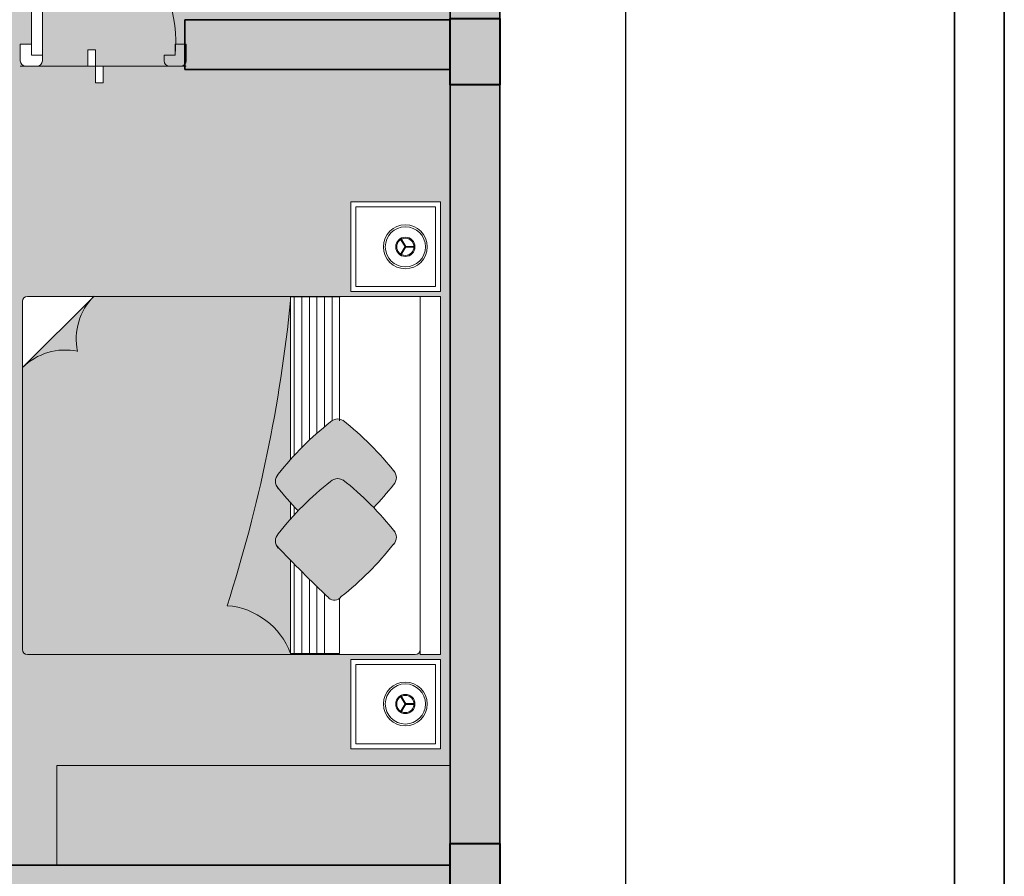
# Model space of a CAD drawing. Units: inches. Extents: x 1077 to 2505, y 1892 to 2728.
# Tile 17 of 26: x 1470 to 1648, y 2431 to 2586. Entities that reach past the tile are written whole.
import ezdxf

# ---------------------------------------------------------------- set-up
doc = ezdxf.new("R2010")
doc.units = ezdxf.units.IN
doc.linetypes.add('ACAD_ISO02W100', pattern=[15, 12, -3])
doc.layers.get('Defpoints').update_dxf_attribs({"color": 220, "linetype": 'ACAD_ISO02W100'})
for name, color, linetype, lineweight in [('00 FURNITURE', 15, 'Continuous', 15), ('A-ANNO-DIMS', 2, 'Continuous', 18), ('A-ANNO-TTLB', 7, 'Continuous', 35), ('A-COLS', 7, 'Continuous', 40), ('A-DOOR', 4, 'Continuous', 18), ('A-FLOR-CASE', 8, 'Continuous', 18), ('A-WALL-PATT', 7, 'Continuous', 9), ('A_FUR 1', 5, 'Continuous', 5), ('WALL', 7, 'Continuous', 35)]:
    doc.layers.add(name, color=color, linetype=linetype, lineweight=lineweight)
for name, color, linetype, lineweight, true_color in [('A-FLOR-CASE-PATT', 32, 'Continuous', 9, 0xcd6928), ('A-FLOR-PATT', 254, 'Continuous', 9, 0xd7ebd2), ('A-FURN-PATT', 177, 'Continuous', 9, 0x293189)]:
    doc.layers.add(name, color=color, linetype=linetype, lineweight=lineweight, true_color=true_color)
doc.styles.get("Standard").update_dxf_attribs({"font": 'arial.ttf'})
doc.dimstyles.get("Standard").update_dxf_attribs({"dimtxt": 10.18, "dimasz": 0.18, "dimexe": 0.18, "dimexo": 0.0625, "dimgap": 0.09, "dimtad": 0, "dimtih": 1, "dimtoh": 1, "dimdec": 0, "dimzin": 0, "dimdsep": 46, "dimlunit": 3, "dimtxsty": 'Standard', "dimcen": 0.09, "dimadec": 0, "dimazin": 0, "dimtfac": 1, "dimtdec": 0, "dimtofl": 0, "dimtmove": 0, "dimatfit": 3, "dimfxl": 1, "dimtolj": 1, "dimtzin": 0, "dimarcsym": 0})

# ---------------------------------------------------------------- blocks, each defined once
blk = doc.blocks.new('ESTSET')
at = {"layer": 'A_FUR 1'}
for p, q in [((-10.44, 4.1), (-10.44, 32.1)), ((-8.44, 4.1), (-8.44, 32.1)), ((-36.44, 6.1), (-36.44, 3.1)), ((-34.44, 6.1), (-36.44, 6.1)), ((-34.44, 4.1), (-34.44, 6.1)), ((-34.44, 4.1), (-34.44, 6.1)), ((-8.44, 4.1), (-8.44, 6.1)), ((-8.44, 6.1), (-6.44, 6.1)), ((-8.44, 4.1), (-8.44, 6.1)), ((-6.44, 6.1), (-6.44, 3.1)), ((-32.44, 4.1), (-34.44, 4.1)), ((-32.44, 4.1), (-34.44, 4.1)), ((-32.44, 3.1), (-32.44, 4.1)), ((-10.44, 3.1), (-10.44, 4.1)), ((-10.44, 4.1), (-8.44, 4.1)), ((-10.44, 4.1), (-8.44, 4.1)), ((-6.44, 2.1), (-36.44, 2.1)), ((-35.44, 2.1), (-33.44, 2.1)), ((-7.44, 2.1), (-9.44, 2.1))]:
    blk.add_line(p, q, dxfattribs=at)
for points in [[(-21.44, 2.1), (-18.67, 2.1), (-18.67, 5.1), (-20.06, 5.1)], [(-20.06, 5.1), (-20.06, -0.91)], [(-21.44, 2.1), (-21.44, -0.91), (-20.06, -0.91)]]:
    blk.add_lwpolyline(points, dxfattribs=at)
for centre, radius, start, end in [((-8.91, 6.46), 25.64, 88.9606, 185.2816), ((-35.44, 3.1), 1, 180, 270), ((-33.44, 3.1), 1, 270, 0), ((-9.44, 3.1), 1, 180, 270), ((-7.44, 3.1), 1, 270, 0)]:
    blk.add_arc(centre, radius, start, end, dxfattribs=at)
blk = doc.blocks.new('RGWTG')
at = {"layer": '00 FURNITURE'}
for p, q in [((578.23, 3473.51), (577.36, 3475.01)), ((578.23, 3473.58), (577.36, 3472.08)), ((578.36, 3473.58), (577.49, 3475.09)), ((578.29, 3473.62), (580.03, 3473.62)), ((578.36, 3473.51), (577.49, 3472)), ((578.29, 3473.47), (580.03, 3473.47)), ((521.93, 3464.58), (509.03, 3451.68)), ((509.03, 3422.63), (509.03, 3463.68)), ((509.93, 3464.58), (566.4, 3464.58)), ((557.53, 3463.84), (557.53, 3464.49)), ((557.53, 3464.49), (566.4, 3464.49)), ((558.2, 3464.49), (558.2, 3435.82)), ((559.57, 3464.49), (559.57, 3437.25)), ((560.94, 3464.49), (560.94, 3438.58)), ((562.3, 3464.49), (562.3, 3439.83)), ((563.67, 3464.49), (563.67, 3440.99)), ((565.04, 3464.49), (565.04, 3442.08)), ((566.4, 3464.58), (580.98, 3464.58)), ((566.4, 3464.49), (566.4, 3442.08)), ((566.4, 3464.49), (566.4, 3463.84)), ((580.98, 3464.58), (580.98, 3416.72)), ((558.2, 3426.48), (558.2, 3425.04)), ((509.03, 3400.68), (509.03, 3422.63)), ((580.98, 3416.72), (580.98, 3400.68)), ((558.2, 3416.13), (558.2, 3399.95)), ((559.57, 3414.75), (559.57, 3399.95)), ((560.94, 3413.39), (560.94, 3399.95)), ((562.3, 3412.04), (562.3, 3399.95)), ((563.67, 3410.72), (563.67, 3399.95)), ((557.53, 3399.95), (557.53, 3400.6)), ((566.4, 3400.6), (566.4, 3399.95)), ((580.08, 3399.78), (509.93, 3399.78)), ((566.4, 3399.95), (557.53, 3399.95)), ((578.23, 3390.78), (577.36, 3392.29)), ((578.36, 3390.86), (577.49, 3392.36)), ((578.23, 3390.86), (577.36, 3389.36)), ((578.36, 3390.78), (577.49, 3389.28)), ((578.29, 3390.9), (580.03, 3390.9)), ((578.29, 3390.74), (580.03, 3390.74))]:
    blk.add_line(p, q, dxfattribs=at)
for points in [[(568.43, 3465.48), (584.63, 3465.48), (584.63, 3481.68), (568.43, 3481.68)], [(569.33, 3466.38), (583.73, 3466.38), (583.73, 3480.78), (569.33, 3480.78)], [(580.98, 3399.78), (584.63, 3399.78), (584.63, 3464.58), (580.98, 3464.58)], [(568.43, 3398.88), (584.63, 3398.88), (584.63, 3382.68), (568.43, 3382.68)], [(569.33, 3397.98), (583.73, 3397.98), (583.73, 3383.58), (569.33, 3383.58)]]:
    blk.add_lwpolyline(points, close=True, dxfattribs=at)
for points in [[(566.52, 3464.49), (557.53, 3464.49), (557.53, 3435.08)], [(557.53, 3427.21), (557.53, 3424.3)], [(557.53, 3416.82), (557.53, 3399.95), (566.4, 3399.95), (566.4, 3409.94)]]:
    blk.add_lwpolyline(points, dxfattribs=at)
for centre, radius in [((578.29, 3473.54), 3.97), ((578.29, 3473.54), 3.63), ((578.29, 3473.54), 1.74), ((578.29, 3473.54), 1.56), ((578.29, 3390.82), 3.97), ((578.29, 3390.82), 3.63), ((578.29, 3390.82), 1.74), ((578.29, 3390.82), 1.56)]:
    blk.add_circle(centre, radius, dxfattribs=at)
for centre, radius, start, end in [((509.93, 3463.68), 0.9, 90, 180), ((529.65, 3456.88), 10.9, 135.0361, 191.9278), ((290.56, 3490.52), 268.3, 342.2214, 354.2925), ((516.73, 3443.97), 10.9, 78.0722, 134.9639), ((598.15, 3399.01), 54.32, 127.931, 142.069), ((566.05, 3440.57), 1.82, 45, 135), ((533.58, 3399.31), 54.32, 37.931, 52.069), ((574.84, 3431.77), 1.82, 315, 45), ((556.59, 3431.11), 1.82, 135, 225), ((598.15, 3388.23), 54.32, 127.931, 142.069), ((566.05, 3429.78), 1.82, 45, 135), ((533.58, 3388.53), 54.32, 37.931, 52.069), ((597.87, 3463.6), 54.32, 217.931, 224.141), ((533.28, 3463.88), 54.32, 316.32, 322.069), ((574.84, 3420.99), 1.82, 315, 45), ((556.59, 3420.33), 1.82, 135, 225), ((765.33, 3619.75), 290.45, 223.6069, 226.2326), ((533.28, 3453.1), 54.32, 307.931, 322.069), ((565.44, 3411.05), 1.47, 225.9674, 326.8337), ((545.02, 3395.29), 13.35, 20.4224, 85.5825), ((509.93, 3400.68), 0.9, 180, 270), ((580.08, 3400.68), 0.9, 270, 0)]:
    blk.add_arc(centre, radius, start, end, dxfattribs=at)
blk = doc.blocks.new('C1')
h = blk.add_hatch(color=256)
h.dxf.hatch_style = 1
h.paths.add_polyline_path([(1668.56, 2445.41), (1677.56, 2445.41), (1677.56, 2457.41), (1668.56, 2457.41)])
for p, q in [((1668.56, 2457.41), (1677.56, 2457.41)), ((1668.56, 2445.41), (1668.56, 2457.41)), ((1677.56, 2457.41), (1677.56, 2445.41)), ((1677.56, 2445.41), (1668.56, 2445.41))]:
    blk.add_line(p, q)
blk = doc.blocks.new('*D14')
at = {"layer": 'A-ANNO-DIMS', "color": 0, "lineweight": -2, "transparency": 16777216}
for p, q in [((1555.59, 2651.66), (1579.43, 2651.66)), ((1579.25, 2651.48), (1579.25, 2375.3)), ((1579.25, 2088.54), (1579.25, 2364.72)), ((1555.59, 2088.36), (1579.43, 2088.36))]:
    blk.add_line(p, q, dxfattribs=at)
at = {"layer": 'A-ANNO-DIMS', "color": 0, "transparency": 16777216}
for points in [[(1579.22, 2651.48), (1579.28, 2651.48), (1579.25, 2651.66)], [(1579.22, 2088.54), (1579.28, 2088.54), (1579.25, 2088.36)]]:
    blk.add_solid(points, dxfattribs=at)
at = {"layer": 'Defpoints', "color": 0, "transparency": 16777216}
for p in [(1555.53, 2651.66), (1555.53, 2088.36), (1579.25, 2088.36)]:
    blk.add_point(p, dxfattribs=at)
at = {"layer": 'A-ANNO-DIMS', "color": 0, "transparency": 16777216, "insert": (1579.25, 2370.01), "char_height": 10.18, "attachment_point": 5}
blk.add_mtext('\\A1;46\'-11"', dxfattribs=at)
blk = doc.blocks.new('SHEET-FRAME-RESIDENTIAL')
for points in [[(0, 830.04), (543.52, 830.04), (543.52, 0), (0, 0)], [(9, 821.04), (534.52, 821.04), (534.52, 9), (9, 9)]]:
    blk.add_lwpolyline(points, close=True)

msp = doc.modelspace()

# ---------------------------------------------------------------- hatches: boundary and pattern name
at = {"layer": 'A-FLOR-CASE-PATT', "transparency": 33554610}
h = msp.add_hatch(color=256, dxfattribs=at)
h.dxf.hatch_style = 1
h.paths.add_polyline_path([(1325.53, 2577.15), (1307.53, 2577.15), (1307.53, 2515.13), (1325.53, 2515.13)])
h.paths.add_polyline_path([(1476.35, 2451.18), (1476.35, 2433.16), (1547.53, 2433.16), (1547.53, 2437.11), (1547.53, 2451.18)])
at = {"layer": 'A-FLOR-PATT', "transparency": 33554559}
h = msp.add_hatch(color=256, dxfattribs=at)
h.dxf.hatch_style = 1
h.paths.add_polyline_path([(1395.53, 2577.16), (1374.83, 2577.16), (1350.83, 2577.19), (1350.83, 2577.16), (1329.53, 2577.16), (1329.53, 2480.16), (1329.53, 2469.16), (1325.53, 2469.16), (1325.53, 2515.13), (1307.53, 2515.13), (1307.53, 2577.16), (1269.31, 2577.16), (1221.31, 2577.15), (1221.31, 2577.16), (1187.53, 2577.16), (1187.53, 2433.16), (1289.53, 2433.16), (1289.53, 2429.16), (1263.53, 2429.16), (1187.53, 2429.16), (1187.53, 2395.02), (1187.53, 2395.02), (1187.53, 2371.02), (1187.53, 2371.02), (1187.53, 2307.16), (1259.53, 2307.16), (1259.53, 2399.16), (1263.53, 2399.16), (1263.53, 2307.16), (1289.53, 2307.16), (1289.53, 2306.23), (1325.53, 2306.23), (1325.53, 2307.16), (1329.53, 2307.16), (1329.53, 2306.23), (1365.53, 2306.23), (1365.53, 2307.16), (1432.53, 2307.16), (1432.53, 2088.16), (1547.53, 2088.16), (1547.53, 2140.08), (1511.53, 2140.08), (1511.53, 2267.16), (1475.53, 2267.16), (1475.53, 2303.16), (1468.53, 2303.16), (1468.53, 2307.16), (1547.53, 2307.16), (1547.53, 2348.22), (1547.53, 2396.22), (1547.53, 2429.16), (1435.53, 2429.16), (1435.53, 2433.16), (1476.35, 2433.16), (1476.35, 2451.18), (1547.53, 2451.18), (1547.53, 2577.16), (1499.53, 2577.16), (1499.53, 2586.16), (1547.53, 2586.16), (1547.53, 2642.16), (1518.18, 2642.16), (1518.18, 2642.05), (1494.15, 2642.05), (1494.15, 2642.16), (1469.53, 2642.16), (1469.53, 2577.16), (1399.53, 2577.16), (1399.53, 2429.16), (1325.53, 2429.16), (1325.53, 2433.16), (1329.53, 2433.16), (1395.53, 2433.16), (1395.53, 2480.16), (1359.53, 2480.16), (1359.53, 2484.16), (1395.53, 2484.16)])
h.paths.add_polyline_path([(1357.65, 2482.07), (1355.65, 2482.07), (1355.65, 2481.07, 0.414214), (1356.65, 2480.07), (1344.65, 2480.07), (1344.65, 2477.06), (1343.27, 2477.06), (1343.27, 2480.07), (1330.65, 2480.07, -0.414214), (1329.65, 2481.07), (1329.65, 2484.07), (1331.65, 2484.07), (1331.65, 2510.07, -0.446908)], flags=16)
h.paths.add_polyline_path([(1305.09, 2559.18), (1288.89, 2559.18), (1288.89, 2575.38), (1305.09, 2575.38)], flags=16)
h.paths.add_polyline_path([(1304.19, 2560.08), (1289.79, 2560.08), (1289.79, 2574.48), (1304.19, 2574.48)], flags=0)
h.paths.add_polyline_path([(1287.99, 2500.68, -0.414214), (1287.09, 2499.78), (1265.14, 2499.78), (1224.09, 2499.78, -0.414214), (1223.19, 2500.68), (1223.19, 2557.16), (1223.19, 2571.74), (1223.19, 2575.38), (1287.99, 2575.38), (1287.99, 2571.74), (1287.09, 2571.74, -0.414214), (1287.99, 2570.84)], flags=16)
h.paths.add_polyline_path([(1292.98, 2569.05, -1), (1300.92, 2569.05, -1)], flags=0)
h.paths.add_polyline_path([(1293.32, 2569.05, -1), (1300.58, 2569.05, -1)], flags=0)
h.paths.add_polyline_path([(1322.8, 2462.21), (1322.8, 2431.71), (1323.05, 2430.71), (1323.05, 2431.71), (1321.8, 2431.71), (1321.8, 2462.19, 0.404641), (1292.3, 2431.71), (1292.05, 2430.71, -0.414214), (1291.55, 2430.21), (1291.05, 2430.21), (1291.05, 2429.71, -0.414214), (1290.55, 2429.21), (1289.55, 2429.21), (1289.55, 2434.21), (1290.55, 2434.21, -0.414214), (1291.05, 2433.71), (1291.05, 2433.21), (1291.55, 2433.21, -0.414214), (1292.05, 2432.71), (1292.3, 2431.71, -0.414214)], flags=16)
h.paths.add_polyline_path([(1287.82, 2548.28, 0.292232), (1279.17, 2536.8, 0.052719), (1223.93, 2548.28), (1223.28, 2548.28), (1223.28, 2557.16), (1223.93, 2557.16), (1245.42, 2557.16, -0.117785), (1245.77, 2557.93, -0.059418), (1254.87, 2567.02, -0.379859), (1257.28, 2566.88, -0.02509), (1261.41, 2563.32, -0.025935), (1265.65, 2567.02, -0.379859), (1268.06, 2566.88, -0.061767), (1277.52, 2557.43, -0.069393), (1277.82, 2557.16), (1287.82, 2557.16)], flags=0)
h.paths.add_polyline_path([(1263.47, 2548.28), (1260.56, 2548.28, -0.015371), (1258.01, 2546.13, -0.429576), (1255.37, 2546.06, -0.016036), (1252.69, 2548.28), (1223.28, 2548.28), (1223.28, 2554.42), (1246.78, 2554.42, 0.055344), (1255.37, 2546.06, 0.331768), (1257.52, 2545.74, 0.027343), (1262, 2549.64, 0.00919)], flags=0)
h.paths.add_polyline_path([(1295.56, 2568.34), (1296.87, 2569.09), (1296.87, 2570.6, 0.399698), (1295.39, 2569.05, 0.119004)], flags=0)
h.paths.add_polyline_path([(1295.21, 2569.05, -1), (1298.68, 2569.05, -1)], flags=0)
h.paths.add_polyline_path([(1296.95, 2568.96), (1297.03, 2569), (1297.03, 2569.09), (1296.99, 2569.11), (1296.91, 2568.98)], flags=0)
h.paths.add_polyline_path([(1402.28, 2462.19, -0.414214), (1432.78, 2431.69), (1433.03, 2432.69), (1432.78, 2431.69, 0.404641), (1403.28, 2462.17), (1403.28, 2431.69), (1402.03, 2431.69), (1402.03, 2430.69, -0.414214), (1401.53, 2430.19), (1401.03, 2430.19), (1401.03, 2429.69, -0.414214), (1400.53, 2429.19), (1399.53, 2429.19), (1399.53, 2434.19), (1400.53, 2434.19, -0.414214), (1401.03, 2433.69), (1401.03, 2433.19), (1401.53, 2433.19, -0.414214), (1402.03, 2432.69)], flags=16)
h.paths.add_polyline_path([(1470.16, 2535.21, -0.414214), (1471.06, 2536.11), (1527.54, 2536.11), (1542.12, 2536.11), (1545.76, 2536.11), (1545.76, 2471.31), (1542.12, 2471.31), (1542.12, 2472.21, -0.414214), (1541.22, 2471.31), (1471.06, 2471.31, -0.414214), (1470.16, 2472.21), (1470.16, 2494.16)], flags=16)
h.paths.add_polyline_path([(1483.07, 2536.11, 0.253465), (1480.11, 2526.15, 0.2538), (1470.15, 2523.19)], flags=16)
h.paths.add_polyline_path([(1223.19, 2512.69, 0.253465), (1233.14, 2509.74, 0.2538), (1236.1, 2499.77)], flags=16)
h.paths.add_polyline_path([(1469.77, 2578.72), (1469.77, 2581.72), (1471.77, 2581.72), (1471.77, 2607.72, -0.01951), (1473.77, 2607.68), (1473.77, 2579.72), (1473.77, 2578.72, -0.414214), (1472.77, 2577.72), (1470.77, 2577.72, -0.414214)], flags=16)
h.paths.add_polyline_path([(1382.46, 2398.13), (1395.04, 2398.13), (1395.04, 2399.74), (1382.46, 2399.74)], flags=16)
h.paths.add_polyline_path([(1379.94, 2397.18), (1379.94, 2389.82), (1380.5, 2389.82), (1380.5, 2396.05, -0.41429), (1381.06, 2396.61), (1396.47, 2396.61, -0.414213), (1397.03, 2396.05), (1397.03, 2389.82), (1397.59, 2389.82), (1397.59, 2397.18)], flags=16)
h.paths.add_polyline_path([(1263.37, 2428.14), (1263.37, 2426.14, -0.414214), (1262.37, 2425.14), (1261.37, 2425.14), (1233.41, 2425.14, 0.400854), (1259.37, 2401.04), (1259.37, 2401.14), (1261.37, 2401.14, -0.446908), (1233.37, 2427.14), (1259.37, 2427.14), (1259.37, 2429.14), (1262.37, 2429.14, -0.414214)], flags=16)
h.paths.add_polyline_path([(1404.79, 2398.13), (1417.37, 2398.13), (1417.37, 2399.74), (1404.79, 2399.74)], flags=16)
h.paths.add_polyline_path([(1402.27, 2397.18), (1404.79, 2398.13), (1417.37, 2398.13), (1419.92, 2397.18)], flags=16)
h.paths.add_polyline_path([(1432.26, 2383.16), (1432.26, 2370.59), (1433.87, 2370.59), (1433.87, 2383.16)], flags=16)
h.paths.add_polyline_path([(1431.3, 2385.69), (1423.84, 2385.69), (1423.84, 2385.13), (1430.18, 2385.13, -0.41429), (1430.74, 2384.57), (1430.74, 2369.16, -0.414237), (1430.18, 2368.6), (1423.84, 2368.6), (1423.84, 2368.03), (1431.3, 2368.03)], flags=16)
h.paths.add_polyline_path([(1417.37, 2351.16), (1417.37, 2349.54), (1418.9, 2349.54, 0.414236), (1419.92, 2350.56), (1419.92, 2352.11)], flags=16)
h.paths.add_polyline_path([(1395.04, 2351.16), (1395.04, 2349.54), (1396.58, 2349.54, 0.414235), (1397.59, 2350.56), (1397.59, 2352.11)], flags=16)
h.paths.add_polyline_path([(1366.7, 2370.05), (1365.09, 2370.05), (1365.09, 2368.52, 0.414235), (1366.11, 2367.5), (1367.66, 2367.5)], flags=16)
h.paths.add_polyline_path([(1419.36, 2359.47), (1419.36, 2353.24, -0.41419), (1418.8, 2352.68), (1403.39, 2352.68, -0.414137), (1402.83, 2353.24), (1402.83, 2359.47), (1397.03, 2359.47), (1397.03, 2353.24, -0.414189), (1396.47, 2352.68), (1381.06, 2352.68, -0.414137), (1380.5, 2353.24), (1380.5, 2359.47)], flags=16)
h.paths.add_polyline_path([(1222.29, 2559.18), (1206.09, 2559.18), (1206.09, 2575.38), (1222.29, 2575.38)], flags=16)
h.paths.add_polyline_path([(1221.39, 2560.08), (1206.99, 2560.08), (1206.99, 2574.48), (1221.39, 2574.48)], flags=0)
h.paths.add_polyline_path([(1482, 2577.72), (1482, 2580.73), (1483.38, 2580.73), (1483.38, 2577.72), (1484.77, 2577.72), (1484.77, 2574.72), (1483.38, 2574.72), (1483.38, 2577.72)], flags=16)
h.paths.add_polyline_path([(1266.37, 2415.53), (1266.37, 2414.14), (1263.37, 2414.14), (1263.37, 2415.53), (1260.36, 2415.53), (1260.36, 2416.91), (1263.37, 2416.91), (1263.37, 2415.53)], flags=16)
h.paths.add_polyline_path([(1210.26, 2569.05, -1), (1218.19, 2569.05, -1)], flags=0)
h.paths.add_polyline_path([(1210.6, 2569.05, -1), (1217.85, 2569.05, -1)], flags=0)
h.paths.add_polyline_path([(1212.84, 2568.34), (1214.15, 2569.09), (1214.15, 2570.6, 0.399698), (1212.67, 2569.05, 0.119004)], flags=0)
h.paths.add_polyline_path([(1212.49, 2569.05, -1), (1215.96, 2569.05, -1)], flags=0)
h.paths.add_polyline_path([(1214.23, 2568.96), (1214.3, 2568.91), (1214.3, 2569)], flags=0)
h.paths.add_polyline_path([(1507.18, 2480.12, 0.052719), (1518.66, 2535.36), (1518.66, 2536.01), (1527.54, 2536.01), (1527.54, 2535.36), (1527.54, 2513.88, -0.117785), (1528.31, 2513.53, -0.059418), (1537.4, 2504.43, -0.379859), (1537.26, 2502.01, -0.02509), (1533.7, 2497.89, -0.025935), (1537.4, 2493.64, -0.379859), (1537.26, 2491.23, -0.061767), (1527.8, 2481.77, -0.069393), (1527.54, 2481.47), (1527.54, 2471.47), (1518.66, 2471.47, 0.292232)], flags=0)
h.paths.add_polyline_path([(1516.43, 2503.92, -0.016036), (1518.66, 2506.6), (1518.66, 2536.01), (1524.8, 2536.01), (1524.8, 2512.51, 0.055344), (1516.43, 2503.92, 0.331768), (1516.12, 2501.77, 0.027343), (1520.01, 2497.29, 0.00919), (1518.66, 2495.82), (1518.66, 2498.73, -0.015371), (1516.5, 2501.28, -0.429576)], flags=0)
h.paths.add_polyline_path([(1499.63, 2625.5, -0.171636), (1502.82, 2631.01), (1502.82, 2633.37), (1498.68, 2633.37, -0.414214), (1497.7, 2634.36), (1497.7, 2640.66, -0.414214), (1498.68, 2641.64), (1514.82, 2641.64, -0.414214), (1515.81, 2640.66), (1515.81, 2634.36, -0.414214), (1514.82, 2633.37), (1510.69, 2633.37), (1510.69, 2631.01, -0.171636), (1513.88, 2625.5, -0.258205), (1509.31, 2614.47), (1504.19, 2614.47, -0.258205)], flags=16)
h.paths.add_polyline_path([(1501.2, 2625.5, -0.171636), (1504.39, 2631.01), (1509.12, 2631.01, -0.171636), (1512.3, 2625.5, -0.210384), (1509.35, 2616.02), (1504.16, 2616.02, -0.210384)], flags=0)
h.paths.add_polyline_path([(1529.56, 2537.01), (1529.56, 2553.21), (1545.76, 2553.21), (1545.76, 2537.01)], flags=16)
h.paths.add_polyline_path([(1530.46, 2537.91), (1530.46, 2552.31), (1544.86, 2552.31), (1544.86, 2537.91)], flags=0)
h.paths.add_polyline_path([(1535.45, 2545.07, -1), (1543.39, 2545.07, -1)], flags=0)
h.paths.add_polyline_path([(1535.8, 2545.07, -1), (1543.05, 2545.07, -1)], flags=0)
h.paths.add_polyline_path([(1529.56, 2470.41), (1545.76, 2470.41), (1545.76, 2454.21), (1529.56, 2454.21)], flags=16)
h.paths.add_polyline_path([(1541.16, 2544.99), (1540.98, 2544.99, -0.544606), (1538.71, 2543.68), (1538.62, 2543.53, 0.547962)], flags=0)
h.paths.add_polyline_path([(1530.46, 2469.51), (1544.86, 2469.51), (1544.86, 2455.11), (1530.46, 2455.11)], flags=0)
h.paths.add_polyline_path([(1539.47, 2545.14), (1539.42, 2545.22), (1539.38, 2545.14)], flags=0)
h.paths.add_polyline_path([(1543.39, 2462.34, -1), (1535.45, 2462.34, -1)], flags=0)
h.paths.add_polyline_path([(1543.05, 2462.34, -1), (1535.8, 2462.34, -1)], flags=0)
h.paths.add_polyline_path([(1541.16, 2462.27), (1540.98, 2462.27, -0.544606), (1538.71, 2460.96), (1538.62, 2460.8, 0.547962)], flags=0)
h.paths.add_polyline_path([(1539.47, 2462.42), (1539.42, 2462.5), (1539.38, 2462.42)], flags=0)
h.paths.add_polyline_path([(1435.32, 2335.25, -0.414214), (1465.82, 2304.75), (1466.07, 2305.75), (1465.82, 2304.75, 0.404641), (1436.32, 2335.23), (1436.32, 2304.75), (1435.07, 2304.75), (1435.07, 2303.75, -0.414214), (1434.57, 2303.25), (1434.07, 2303.25), (1434.07, 2302.75, -0.414214), (1433.57, 2302.25), (1432.57, 2302.25), (1432.57, 2307.25), (1433.57, 2307.25, -0.414214), (1434.07, 2306.75), (1434.07, 2306.25), (1434.57, 2306.25, -0.414214), (1435.07, 2305.75)], flags=16)
h.paths.add_polyline_path([(1532.13, 2635.71), (1535.43, 2635.71), (1535.43, 2635.89), (1532.13, 2635.89)], flags=16)
edge = h.paths.add_edge_path(flags=16)
edge.add_arc((1535.98, 2632.67), 0.183, 270, 360)
edge.add_line((1536.17, 2632.67), (1536.17, 2639.82))
edge.add_line((1536.17, 2639.82), (1538.29, 2639.82))
edge.add_line((1538.29, 2639.82), (1538.29, 2641.82))
edge.add_line((1538.29, 2641.82), (1533.25, 2641.82))
edge.add_line((1533.25, 2641.82), (1533.25, 2639.82))
edge.add_line((1533.25, 2639.82), (1534.87, 2639.82))
edge.add_line((1534.87, 2639.82), (1534.87, 2639))
edge.add_line((1534.87, 2639), (1533.7, 2639))
edge.add_line((1533.7, 2639), (1533.7, 2639.82))
edge.add_line((1533.7, 2639.82), (1533.25, 2639.82))
edge.add_line((1533.25, 2639.82), (1533.25, 2641.82))
edge.add_line((1533.25, 2641.82), (1538.29, 2641.82))
edge.add_line((1538.29, 2641.82), (1538.29, 2641.34))
edge.add_line((1538.29, 2641.34), (1540.64, 2641.58))
edge.add_line((1540.64, 2641.58), (1540.64, 2641.82))
edge.add_line((1540.64, 2641.82), (1541.5, 2641.82))
edge.add_line((1541.5, 2641.82), (1541.5, 2641.25))
edge.add_line((1541.5, 2641.25), (1541.31, 2639.79))
edge.add_ellipse((1541.09, 2638.95), major_axis=(-1.08, 0), ratio=0.790849, start_angle=180, end_angle=255.2976, ccw=False)
edge.add_line((1542.17, 2638.95), (1542.17, 2638.38))
edge.add_ellipse((1541.09, 2638.38), major_axis=(-1.08, 0), ratio=0.790849, start_angle=0, end_angle=180, ccw=False)
edge.add_line((1540, 2638.38), (1540.01, 2638.87))
edge.add_ellipse((1541.09, 2638.95), major_axis=(-1.08, 0), ratio=0.790849, start_angle=284.7024, end_angle=364.0401, ccw=False)
edge.add_line((1540.78, 2639.75), (1540.78, 2641.25))
edge.add_line((1540.78, 2641.25), (1540.64, 2641.25))
edge.add_line((1540.64, 2641.25), (1538.29, 2641.01))
edge.add_line((1538.29, 2641.01), (1538.29, 2639.82))
edge.add_line((1538.29, 2639.82), (1536.17, 2639.82))
edge.add_line((1536.17, 2639.82), (1536.17, 2632.48))
edge.add_line((1536.17, 2632.48), (1535.98, 2632.48))
h.paths.add_polyline_path([(1496.32, 2250.34, -0.292371), (1498.9, 2247.83, -0.085148), (1501.21, 2208.85, -0.01331), (1500.27, 2098.5, -0.379287), (1497.22, 2095.28, -0.0502), (1441.54, 2095.28, -0.379287), (1438.5, 2098.5, -0.01331), (1437.56, 2208.85, -0.086132), (1439.96, 2248.26, -0.295116), (1442.59, 2250.78, -0.114238)], flags=16)
h.paths.add_polyline_path([(1495.16, 2205.84, -0.355389), (1496.7, 2202.1), (1492.94, 2189.65, -0.398275), (1489.12, 2187.47, 0.113332), (1449.64, 2187.47, -0.398275), (1445.82, 2189.65), (1442.06, 2202.1, -0.355394), (1443.6, 2205.84, -0.265725)], flags=0)
h.paths.add_polyline_path([(1440.37, 2195.72), (1445.94, 2181.67), (1445.94, 2160.63), (1440.84, 2157.26)], flags=0)
h.paths.add_polyline_path([(1498.46, 2195.72), (1497.99, 2157.26), (1492.88, 2160.63), (1492.88, 2181.67)], flags=0)
h.paths.add_polyline_path([(1445.94, 2158.37), (1445.94, 2137.12), (1441.12, 2122.56), (1440.87, 2155.03)], flags=0)
h.paths.add_polyline_path([(1492.88, 2158.37), (1497.96, 2155.03), (1497.71, 2122.56), (1492.88, 2137.12)], flags=0)
h.paths.add_polyline_path([(1489.88, 2130.4), (1494.39, 2107.67, -0.090102), (1444.44, 2107.65), (1448.95, 2130.39, 0.036636)], flags=0)
h.paths.add_polyline_path([(1447.54, 2159.34), (1497.44, 2159.34), (1497.44, 2177.89), (1447.54, 2177.89)], flags=8)
h.paths.add_polyline_path([(1196.44, 2354.84), (1246.65, 2354.84), (1246.65, 2388.43), (1196.44, 2388.43)], flags=24)
h.paths.add_polyline_path([(1296.09, 2360.25), (1353.81, 2360.25), (1353.81, 2393.84), (1296.09, 2393.84)], flags=24)
h.paths.add_polyline_path([(1400.72, 2471.85), (1470.63, 2471.85), (1470.63, 2505.44), (1400.72, 2505.44)], flags=24)
h.paths.add_polyline_path([(1324.78, 2448.48), (1394.95, 2448.48), (1394.95, 2467.02), (1324.78, 2467.02)], flags=24)
h.paths.add_polyline_path([(1335.08, 2531.43), (1389.67, 2531.43), (1389.67, 2565.02), (1335.08, 2565.02)], flags=24)
h.paths.add_polyline_path([(1225.76, 2460), (1295.67, 2460), (1295.67, 2493.58), (1225.76, 2493.58)], flags=24)
h = msp.add_hatch(color=256, dxfattribs=at)
h.dxf.hatch_style = 1
h.paths.add_polyline_path([(1547.53, 2348.22), (1547.53, 2396.22), (1547.53, 2425.11), (1547.53, 2425.11), (1547.53, 2429.16), (1435.53, 2429.16), (1434.03, 2429.21), (1434.03, 2430.19), (1433.03, 2430.19), (1432.78, 2431.69, 0.404641), (1403.28, 2462.17), (1403.28, 2431.69), (1402.03, 2431.69), (1402.03, 2430.19), (1401.03, 2430.19), (1401.03, 2429.19), (1399.53, 2429.19), (1399.53, 2429.19), (1399.53, 2429.16), (1334.67, 2429.16), (1334.67, 2423.95), (1325.67, 2423.95), (1325.67, 2429.16), (1325.53, 2429.16), (1324.05, 2429.24), (1324.05, 2430.21), (1323.05, 2430.21), (1323.05, 2431.71), (1321.8, 2431.71), (1321.8, 2462.19, 0.416544), (1292.05, 2430.73, -0.423614), (1291.55, 2430.21), (1291.05, 2430.21), (1291.05, 2429.21), (1289.55, 2429.21), (1289.53, 2429.21), (1289.53, 2429.16), (1263.37, 2429.16), (1263.37, 2415.53), (1266.37, 2415.53), (1266.37, 2414.14), (1263.37, 2414.14), (1263.37, 2399.16), (1263.53, 2399.16), (1263.53, 2307.16), (1289.53, 2307.16), (1289.53, 2306.23), (1323.26, 2306.23), (1323.26, 2307.21), (1332.26, 2307.21), (1365.53, 2306.23), (1365.53, 2307.16), (1432.53, 2307.16), (1432.57, 2307.16), (1432.57, 2307.25), (1434.07, 2307.25), (1434.07, 2306.25), (1435.32, 2306.25), (1435.32, 2335.25, -0.407346), (1466.07, 2305.73, -0.423614), (1466.57, 2306.25), (1467.07, 2306.25), (1467.07, 2307.25), (1468.57, 2307.25), (1547.53, 2307.16), (1547.53, 2307.2)])
h.paths.add_polyline_path([(1430.74, 2369.16), (1430.74, 2384.57, 0.41429), (1430.18, 2385.13), (1423.84, 2385.13), (1423.84, 2368.6), (1430.18, 2368.6, 0.414237)], flags=16)
h.paths.add_polyline_path([(1432.26, 2383.16), (1432.26, 2370.59), (1433.87, 2370.59), (1433.87, 2383.16)], flags=16)
h.paths.add_polyline_path([(1431.3, 2368.03), (1431.3, 2385.69), (1432.26, 2383.16), (1432.26, 2370.59)], flags=16)
h.paths.add_polyline_path([(1417.37, 2351.16), (1417.37, 2349.54), (1418.9, 2349.54, 0.414236), (1419.92, 2350.56), (1419.92, 2352.11)], flags=16)
h.paths.add_polyline_path([(1403.39, 2352.68), (1418.78, 2352.68, 0.42427), (1419.36, 2353.24), (1419.36, 2359.47), (1402.83, 2359.47), (1402.83, 2353.24, 0.414137)], flags=16)
h.paths.add_polyline_path([(1366.7, 2370.05), (1365.09, 2370.05), (1365.09, 2368.52, 0.414235), (1366.11, 2367.5), (1367.66, 2367.5)], flags=16)
h.paths.add_polyline_path([(1382.46, 2398.13), (1395.04, 2398.13), (1395.04, 2399.74), (1382.46, 2399.74)], flags=16)
h.paths.add_polyline_path([(1396.47, 2396.61), (1381.06, 2396.61, 0.41429), (1380.5, 2396.05), (1380.5, 2389.82), (1397.03, 2389.82), (1397.03, 2396.05, 0.414213)], flags=16)
h.paths.add_polyline_path([(1402.27, 2397.18), (1402.83, 2396.05, -0.414213), (1403.39, 2396.61)], flags=16)
h.paths.add_polyline_path([(1418.8, 2396.61), (1419.36, 2396.61), (1419.36, 2396.05, 0.414237)], flags=16)
h.paths.add_polyline_path([(1404.79, 2398.13), (1417.37, 2398.13), (1417.37, 2399.74), (1404.79, 2399.74)], flags=16)
h.paths.add_polyline_path([(1381.06, 2352.68, -0.414213), (1380.5, 2353.24), (1380.27, 2352.11)], flags=16)
h.paths.add_polyline_path([(1396.58, 2349.54), (1396.58, 2349.54), (1395.04, 2349.54), (1395.04, 2349.54), (1382.46, 2349.54), (1382.46, 2351.16), (1395.04, 2351.16), (1397.59, 2352.11), (1397.59, 2350.56, -0.414235)], flags=16)
h.paths.add_polyline_path([(1379.94, 2397.18), (1382.46, 2398.13), (1395.04, 2398.13), (1397.59, 2397.18)], flags=16)
h.paths.add_polyline_path([(1368.78, 2384.59, 0.414213), (1368.22, 2384.03), (1367.66, 2367.5), (1367.66, 2385.15)], flags=16)
h.paths.add_polyline_path([(1547.53, 2574.38), (1547.51, 2574.38), (1547.51, 2577.16), (1499.53, 2577.16), (1484.77, 2577.44), (1484.77, 2574.72), (1483.38, 2574.72), (1483.38, 2577.72), (1482, 2577.72), (1469.53, 2577.72), (1469.53, 2577.16), (1401.95, 2577.16), (1401.95, 2574.12), (1399.53, 2574.12), (1399.53, 2434.19), (1401.03, 2434.19), (1401.03, 2433.19), (1402.28, 2433.19), (1402.28, 2462.19, -0.407346), (1433.03, 2432.67, -0.423614), (1433.53, 2433.19), (1434.03, 2433.19), (1434.03, 2434.19), (1435.53, 2434.19), (1476.35, 2433.81), (1476.35, 2451.18), (1547.53, 2451.18)])
h.paths.add_polyline_path([(1470.16, 2535.21, -0.414214), (1471.06, 2536.11), (1527.54, 2536.11), (1542.12, 2536.11), (1545.76, 2536.11), (1545.76, 2471.31), (1542.12, 2471.31), (1542.12, 2472.21, -0.414214), (1541.22, 2471.31), (1471.06, 2471.31, -0.414214), (1470.16, 2472.21), (1470.16, 2494.16)], flags=16)
h.paths.add_polyline_path([(1483.07, 2536.11, 0.253465), (1480.11, 2526.15, 0.2538), (1470.15, 2523.19)], flags=16)
h.paths.add_polyline_path([(1525.55, 2481.52, -0.000893), (1524.8, 2482.24), (1524.8, 2471.47), (1527.54, 2471.47), (1527.54, 2472.12), (1527.54, 2481.47, -0.388819)], flags=0)
h.paths.add_polyline_path([(1518.66, 2536.01), (1527.54, 2536.01), (1527.54, 2535.36), (1527.54, 2513.88, -0.117785), (1528.31, 2513.53, -0.059418), (1537.4, 2504.43, -0.379859), (1537.26, 2502.01, -0.02509), (1533.7, 2497.89, 0.033431), (1528.3, 2502.74, 0.308459), (1526.25, 2502.88, 0.047827), (1518.66, 2495.82), (1518.66, 2498.73, -0.015371), (1516.5, 2501.28, -0.429576), (1516.43, 2503.92, -0.016036), (1518.66, 2506.6)], flags=0)
h.paths.add_polyline_path([(1529.56, 2537.01), (1529.56, 2553.21), (1545.76, 2553.21), (1545.76, 2537.01)], flags=16)
h.paths.add_polyline_path([(1530.46, 2537.91), (1530.46, 2552.31), (1544.86, 2552.31), (1544.86, 2537.91)], flags=0)
h.paths.add_polyline_path([(1535.8, 2545.07, -1), (1543.05, 2545.07, -1)], flags=0)
h.paths.add_polyline_path([(1541.16, 2544.99), (1540.98, 2544.99, -0.544606), (1538.71, 2543.68), (1538.62, 2543.53, 0.547962)], flags=0)
h.paths.add_polyline_path([(1539.47, 2545.14), (1539.42, 2545.22), (1539.38, 2545.14)], flags=0)
h.paths.add_polyline_path([(1529.56, 2470.41), (1545.76, 2470.41), (1545.76, 2454.21), (1529.56, 2454.21)], flags=16)
h.paths.add_polyline_path([(1530.46, 2469.51), (1544.86, 2469.51), (1544.86, 2455.11), (1530.46, 2455.11)], flags=0)
h.paths.add_polyline_path([(1535.8, 2462.34, -1), (1543.05, 2462.34, -1)], flags=0)
h.paths.add_polyline_path([(1541.16, 2462.27), (1540.98, 2462.27, -0.544606), (1538.71, 2460.96), (1538.62, 2460.8, 0.547962)], flags=0)
h.paths.add_polyline_path([(1539.47, 2462.42), (1539.42, 2462.5), (1539.38, 2462.42)], flags=0)
h.paths.add_polyline_path([(1395.53, 2574.12), (1392.95, 2574.12), (1392.95, 2577.16), (1374.83, 2577.16), (1350.83, 2577.19), (1350.83, 2577.16), (1332.07, 2577.16), (1332.07, 2574), (1329.53, 2574), (1329.53, 2484.07), (1331.65, 2484.07), (1331.65, 2510.07, -0.423677), (1357.76, 2484.07), (1359.53, 2484.07), (1359.53, 2484.16), (1395.53, 2484.16)], flags=17)
h.paths.add_polyline_path([(1395.53, 2480.16), (1359.06, 2480.16, 0.437533), (1359.53, 2481.55), (1359.53, 2484.16), (1395.53, 2484.16), (1395.53, 2574.12), (1392.95, 2574.12), (1392.95, 2577.16), (1374.83, 2577.16), (1350.83, 2577.19), (1350.83, 2577.16), (1332.07, 2577.16), (1332.07, 2574), (1329.53, 2574), (1329.53, 2484.07), (1329.65, 2484.07), (1329.65, 2481.07), (1329.53, 2480.16), (1329.53, 2469.16), (1325.53, 2469.16), (1325.53, 2515.13), (1307.53, 2515.13), (1307.53, 2577.16), (1269.31, 2577.16), (1221.31, 2577.15), (1221.31, 2577.16), (1187.61, 2577.16), (1187.61, 2574.03), (1187.53, 2433.16), (1289.55, 2433.16), (1289.55, 2434.21), (1291.05, 2434.21), (1291.05, 2433.21), (1292.05, 2433.21), (1292.3, 2431.71, -0.414214), (1322.8, 2462.21), (1323.05, 2432.71, -0.414214), (1323.55, 2433.21), (1324.05, 2433.21), (1324.05, 2434.21), (1325.67, 2434.21), (1325.67, 2435.95), (1334.67, 2435.95), (1334.67, 2433.16), (1395.53, 2433.16)])
h.paths.add_polyline_path([(1344.65, 2480.07), (1344.65, 2477.06), (1343.27, 2477.06), (1343.27, 2480.07), (1332.65, 2480.07, 0.414214), (1333.65, 2481.07), (1333.65, 2482.07), (1331.65, 2482.07), (1331.65, 2484.07), (1331.65, 2510.07, -0.446908), (1357.65, 2482.07), (1355.65, 2482.07), (1355.65, 2481.07, 0.414214), (1356.65, 2480.07)], flags=16)
h.paths.add_polyline_path([(1287.99, 2500.68, -0.414214), (1287.09, 2499.78), (1265.14, 2499.78), (1224.09, 2499.78, -0.414214), (1223.19, 2500.68), (1223.19, 2557.16), (1223.19, 2571.74), (1223.19, 2575.38), (1287.99, 2575.38), (1287.99, 2571.74), (1287.09, 2571.74, -0.414214), (1287.99, 2570.84)], flags=16)
h.paths.add_polyline_path([(1277.77, 2555.17, -0.000893), (1277.05, 2554.42), (1287.82, 2554.42), (1287.82, 2557.16), (1287.17, 2557.16), (1277.82, 2557.16, -0.388819)], flags=0)
h.paths.add_polyline_path([(1223.28, 2548.28), (1223.28, 2557.16), (1223.93, 2557.16), (1245.42, 2557.16, -0.117785), (1245.77, 2557.93, -0.059418), (1254.87, 2567.02, -0.379859), (1257.28, 2566.88, -0.02509), (1261.41, 2563.32, 0.033431), (1256.55, 2557.93, 0.308459), (1256.41, 2555.88, 0.047827), (1263.47, 2548.28), (1260.56, 2548.28, -0.015371), (1258.01, 2546.13, -0.429576), (1255.37, 2546.06, -0.016036), (1252.69, 2548.28)], flags=0)
h.paths.add_polyline_path([(1305.09, 2559.18), (1288.89, 2559.18), (1288.89, 2575.38), (1305.09, 2575.38)], flags=16)
h.paths.add_polyline_path([(1304.19, 2560.08), (1289.79, 2560.08), (1289.79, 2574.48), (1304.19, 2574.48)], flags=0)
h.paths.add_polyline_path([(1300.58, 2569.05, -1), (1293.32, 2569.05, -1)], flags=0)
h.paths.add_polyline_path([(1223.19, 2512.69, 0.253465), (1233.14, 2509.74, 0.2538), (1236.1, 2499.77)], flags=16)
h.paths.add_polyline_path([(1295.56, 2568.34), (1296.87, 2569.09), (1296.87, 2570.6, 0.399698), (1295.39, 2569.05, 0.119004)], flags=0)
h.paths.add_polyline_path([(1295.21, 2569.05, -1), (1298.68, 2569.05, -1)], flags=0)
h.paths.add_polyline_path([(1296.95, 2568.96), (1297.03, 2569), (1297.03, 2569.09), (1296.99, 2569.11), (1296.91, 2568.98)], flags=0)
h.paths.add_polyline_path([(1222.29, 2559.18), (1206.09, 2559.18), (1206.09, 2575.38), (1222.29, 2575.38)], flags=16)
h.paths.add_polyline_path([(1221.39, 2560.08), (1206.99, 2560.08), (1206.99, 2574.48), (1221.39, 2574.48)], flags=0)
h.paths.add_polyline_path([(1217.85, 2569.05, -1), (1210.6, 2569.05, -1)], flags=0)
h.paths.add_polyline_path([(1212.84, 2568.34), (1214.15, 2569.09), (1214.15, 2570.6, 0.399698), (1212.67, 2569.05, 0.119004)], flags=0)
h.paths.add_polyline_path([(1212.49, 2569.05, -1), (1215.96, 2569.05, -1)], flags=0)
h.paths.add_polyline_path([(1214.23, 2568.96), (1214.3, 2569), (1214.3, 2569.09), (1214.26, 2569.11), (1214.19, 2568.98)], flags=0)
h.paths.add_polyline_path([(1259.53, 2399.14), (1259.37, 2399.14), (1259.37, 2401.04, -0.423677), (1233.37, 2427.14), (1259.37, 2427.14), (1259.37, 2429.16), (1187.53, 2429.16), (1187.53, 2395.02), (1187.53, 2395.02), (1187.53, 2371.02), (1187.53, 2371.02), (1187.53, 2311.49), (1187.55, 2311.49), (1187.55, 2307.16), (1259.53, 2307.16)])
h.paths.add_polyline_path([(1323.26, 2295.21), (1323.26, 2304.23), (1289.53, 2304.23), (1289.53, 2303.16), (1187.55, 2303.16), (1187.55, 2299.49), (1178.53, 2299.49), (1178.53, 2267.66), (1178.53, 2219.66), (1182.03, 2219.66), (1182.03, 2267.67), (1184.03, 2267.67), (1184.03, 2219.66), (1187.53, 2219.66), (1187.53, 2153.16), (1228.13, 2153.16), (1276.13, 2153.16), (1276.13, 2153.16), (1324.54, 2153.16), (1324.54, 2154.67), (1325.54, 2154.67), (1325.54, 2155.92), (1296.54, 2155.92, -0.407346), (1326.06, 2186.67, -0.423614), (1325.54, 2187.17), (1325.54, 2187.67), (1324.54, 2187.67), (1324.54, 2189.17), (1325.43, 2295.21)])
h.paths.add_polyline_path([(1432.53, 2307.16), (1365.53, 2307.16), (1365.53, 2306.23), (1365.53, 2303.16), (1428.53, 2303.16), (1428.53, 2221.2), (1428.57, 2221.2), (1428.57, 2197.2), (1428.53, 2197.16), (1428.53, 2303.01), (1404.46, 2303.01), (1404.46, 2221.2), (1329.53, 2221.2), (1329.53, 2307.16), (1325.53, 2307.16), (1325.53, 2295.21), (1325.43, 2295.21), (1324.54, 2189.17), (1324.54, 2187.67), (1326.04, 2187.67, 1.016365), (1326.06, 2186.67, 0.407348), (1296.54, 2155.92), (1325.54, 2155.92), (1325.54, 2154.67), (1324.54, 2154.67), (1324.54, 2153.16), (1329.53, 2153.16), (1329.53, 2144.16), (1432.53, 2144.16)])
h.paths.add_polyline_path([(1361.95, 2194.26), (1361.95, 2193.16), (1329.53, 2193.16), (1329.53, 2189.16), (1329.54, 2188.17), (1329.54, 2189.16), (1329.53, 2189.16), (1329.53, 2193.16), (1361.95, 2193.16), (1361.95, 2196.26), (1409.95, 2196.26), (1409.95, 2194.26)], flags=16)
h.paths.add_polyline_path([(1377.02, 2200.5), (1345.91, 2200.5), (1345.91, 2218.4), (1347.87, 2218.4), (1347.87, 2219.18), (1374.75, 2219.18), (1374.75, 2218.4), (1377.02, 2218.4)], flags=16)
h.paths.add_polyline_path([(1367.07, 2210.7, -1), (1373.34, 2210.7, -1)], flags=0)
h.paths.add_polyline_path([(1349.92, 2210.7, -1), (1356.98, 2210.7, -1)], flags=0)
h.paths.add_polyline_path([(1405.95, 2256.57), (1405.95, 2277.6), (1427.86, 2277.6), (1427.86, 2256.57)], flags=16)
h.paths.add_polyline_path([(1412.92, 2258.68, -0.414201), (1410.93, 2260.67), (1410.93, 2273.62, -0.414239), (1412.92, 2275.61), (1423.88, 2275.61, -0.414227), (1425.87, 2273.62), (1425.87, 2260.67, -0.414214), (1423.88, 2258.68)], flags=0)
h.paths.add_polyline_path([(1407.61, 2263.66, -1), (1409.18, 2263.66, -1)], flags=0)
h.paths.add_polyline_path([(1407.61, 2267.14, -1), (1409.18, 2267.14, -1)], flags=0)
h.paths.add_polyline_path([(1416.91, 2267.15, -1), (1419.89, 2267.15, -1)], flags=0)
h.paths.add_polyline_path([(1407.61, 2270.63, -1), (1409.18, 2270.63, -1)], flags=0)
h.paths.add_polyline_path([(1475.53, 2303.16), (1468.57, 2303.16), (1468.57, 2302.25), (1467.07, 2302.25), (1467.07, 2303.25), (1466.07, 2303.25), (1465.82, 2304.75, 0.404641), (1436.32, 2335.23), (1436.32, 2304.75), (1435.07, 2304.75), (1435.07, 2303.25), (1434.07, 2303.25), (1434.07, 2302.25), (1432.53, 2302.25), (1432.53, 2144.16), (1432.53, 2088.16), (1547.52, 2088.16), (1547.52, 2100.19), (1547.52, 2140.08), (1511.53, 2140.08), (1511.53, 2267.16), (1475.53, 2267.16)])
h.paths.add_polyline_path([(1438.35, 2102.86, 0.033498), (1438.37, 2102.21, -0.000079)], flags=16)
h.paths.add_polyline_path([(1496.32, 2250.34, -0.292371), (1498.9, 2247.83, -0.085148), (1501.21, 2208.85, -0.012784), (1500.42, 2102.86, -0.033498), (1500.39, 2102.21, 0.012863), (1501.21, 2208.85, 0.077283), (1499.67, 2244.3, 0.265882), (1497.48, 2246.8, 0.14401), (1441.46, 2247.36, 0.270646), (1439.21, 2244.85, -0.007564), (1439.96, 2248.26, -0.295116), (1442.59, 2250.78, -0.114238)], flags=16)
h.paths.add_polyline_path([(1495.16, 2205.84, -0.355389), (1496.7, 2202.1), (1492.94, 2189.65, -0.398275), (1489.12, 2187.47, 0.113332), (1449.64, 2187.47, -0.398275), (1445.82, 2189.65), (1442.06, 2202.1, -0.355394), (1443.6, 2205.84, -0.265725)], flags=16)
h.paths.add_polyline_path([(1440.37, 2195.72), (1445.94, 2181.67), (1445.94, 2160.63), (1440.84, 2157.26)], flags=16)
h.paths.add_polyline_path([(1498.46, 2195.72), (1497.99, 2157.26), (1492.88, 2160.63), (1492.88, 2181.67)], flags=16)
h.paths.add_polyline_path([(1445.94, 2158.37), (1445.94, 2137.12), (1441.12, 2122.56), (1440.87, 2155.03)], flags=16)
h.paths.add_polyline_path([(1492.88, 2158.37), (1497.96, 2155.03), (1497.71, 2122.56), (1492.88, 2137.12)], flags=16)
h.paths.add_polyline_path([(1489.88, 2130.4), (1494.39, 2107.67, -0.090102), (1444.44, 2107.65), (1448.95, 2130.39, 0.036636)], flags=16)
h.paths.add_polyline_path([(1296.09, 2360.25), (1353.81, 2360.25), (1353.81, 2393.84), (1296.09, 2393.84)], flags=24)
h.paths.add_polyline_path([(1400.72, 2471.85), (1470.63, 2471.85), (1470.63, 2505.44), (1400.72, 2505.44)], flags=24)
h.paths.add_polyline_path([(1335.08, 2531.43), (1389.67, 2531.43), (1389.67, 2565.02), (1335.08, 2565.02)], flags=24)
h.paths.add_polyline_path([(1324.78, 2448.48), (1394.95, 2448.48), (1394.95, 2467.02), (1324.78, 2467.02)], flags=24)
h.paths.add_polyline_path([(1225.76, 2460), (1295.67, 2460), (1295.67, 2493.58), (1225.76, 2493.58)], flags=24)
h.paths.add_polyline_path([(1196.44, 2354.84), (1246.65, 2354.84), (1246.65, 2388.43), (1196.44, 2388.43)], flags=24)
h.paths.add_polyline_path([(1447.54, 2159.34), (1497.44, 2159.34), (1497.44, 2177.89), (1447.54, 2177.89)], flags=24)
at = {"layer": 'A-FURN-PATT', "transparency": 33554610}
h = msp.add_hatch(color=256, dxfattribs=at)
h.dxf.hatch_style = 1
h.paths.add_polyline_path([(1518.66, 2535.36), (1518.66, 2536.11), (1483.07, 2536.11, 0.253465), (1480.11, 2526.15, 0.253465), (1470.16, 2523.2), (1470.16, 2494.16), (1470.16, 2472.21, 0.414214), (1471.06, 2471.31), (1518.72, 2471.31, 0.295777), (1507.18, 2480.12, 0.052719)])
h.paths.add_polyline_path([(1483.07, 2536.11), (1470.15, 2523.19, -0.2538), (1480.11, 2526.15, -0.253465)])
h.paths.add_polyline_path([(1528.3, 2502.74, 0.379859), (1525.89, 2502.6, 0.061767), (1516.43, 2493.14, 0.334836), (1516.13, 2490.97, 0.011497), (1525.56, 2481.51, 0.468078), (1527.8, 2481.77, 0.061767), (1537.26, 2491.23, 0.380465), (1537.4, 2493.65, 0.059418)])
h.paths.add_polyline_path([(1528.3, 2513.52, 0.379859), (1525.89, 2513.38, 0.061767), (1516.43, 2503.92, 0.331768), (1516.12, 2501.77, 0.027343), (1520.01, 2497.29, -0.036481), (1525.89, 2502.6, -0.379859), (1528.3, 2502.74, -0.033431), (1533.69, 2497.88, 0.025099), (1537.26, 2502.01, 0.380465), (1537.4, 2504.43, 0.059418)])
h.paths.add_polyline_path([(1518.66, 2488.34, -0.003141), (1516.13, 2490.97, -0.334836), (1516.43, 2493.14, -0.016036), (1518.66, 2495.82), (1518.66, 2498.73, -0.015371), (1516.5, 2501.28, -0.429576), (1516.43, 2503.92, -0.016036), (1518.66, 2506.6), (1518.66, 2535.36, -0.052719), (1507.18, 2480.12, -0.292232), (1518.66, 2471.47)], flags=17)
at = {"layer": 'A-WALL-PATT', "transparency": 33554585}
h = msp.add_hatch(color=256, dxfattribs=at)
h.dxf.hatch_style = 1
h.paths.add_polyline_path([(1187.53, 2424), (1178.53, 2424), (1178.53, 2395.02), (1187.53, 2395.02)])
h.paths.add_polyline_path([(1187.53, 2371.02), (1178.53, 2371.02), (1178.53, 2311.49), (1187.53, 2311.49)])
h.paths.add_polyline_path([(1228.13, 2153.16), (1187.53, 2153.16), (1187.53, 2219.66), (1178.53, 2219.66), (1178.53, 2100.18), (1187.53, 2100.18), (1187.53, 2144.16), (1228.13, 2144.16)])
h.paths.add_polyline_path([(1432.53, 2097.16), (1187.53, 2097.16), (1187.53, 2100.18), (1178.53, 2100.18), (1178.53, 2088.16), (1432.53, 2088.16)])
h.paths.add_polyline_path([(1556.53, 2348.22), (1547.53, 2348.22), (1547.53, 2348.22), (1547.53, 2307.16), (1468.53, 2307.16), (1468.53, 2303.16), (1547.53, 2303.16), (1547.53, 2088.16), (1556.53, 2088.16)])
h.paths.add_polyline_path([(1556.53, 2425.11), (1547.53, 2425.11), (1547.53, 2396.22), (1556.53, 2396.22)])
h.paths.add_polyline_path([(1547.53, 2433.16), (1435.53, 2433.16), (1435.53, 2429.16), (1547.53, 2429.16)])
h.paths.add_polyline_path([(1556.53, 2574.38), (1547.53, 2574.38), (1547.53, 2451.18), (1547.55, 2451.18), (1547.55, 2437.11), (1556.53, 2437.11)])
h.paths.add_polyline_path([(1556.53, 2639.11), (1547.53, 2639.11), (1547.53, 2586.38), (1556.53, 2586.38)])
h.paths.add_polyline_path([(1556.53, 2639.11), (1547.53, 2639.11), (1547.53, 2642.16), (1518.18, 2642.16), (1518.18, 2642.05), (1494.18, 2642.05), (1494.18, 2651.05), (1518.15, 2651.05), (1518.15, 2651.16), (1556.53, 2651.16)])
h.paths.add_polyline_path([(1494.15, 2651.16), (1469.6, 2651.16), (1469.6, 2642.16), (1494.15, 2642.16)])
h.paths.add_polyline_path([(1221.31, 2577.16), (1187.61, 2577.16), (1187.61, 2574.03), (1178.61, 2574.03), (1178.61, 2586.16), (1221.31, 2586.16)])
h.paths.add_polyline_path([(1323.07, 2586.16), (1269.31, 2586.16), (1269.31, 2577.16), (1323.07, 2577.16)])
h.paths.add_polyline_path([(1374.84, 2586.19), (1374.84, 2577.19), (1350.84, 2577.19), (1350.83, 2577.19), (1350.83, 2577.16), (1332.07, 2577.16), (1332.07, 2574), (1323.07, 2574), (1323.07, 2586.16), (1350.83, 2586.16), (1350.84, 2586.16), (1350.84, 2586.19)])
h.paths.add_polyline_path([(1392.95, 2586.16), (1374.84, 2586.16), (1374.84, 2577.16), (1392.95, 2577.16)], flags=17)
h.paths.add_polyline_path([(1469.53, 2642.16), (1469.6, 2651.16), (1460.53, 2651.16), (1460.53, 2586.16), (1392.95, 2586.16), (1392.95, 2577.16), (1395.53, 2577.16), (1395.53, 2484.16), (1359.53, 2484.16), (1359.53, 2480.16), (1395.53, 2480.16), (1395.53, 2433.16), (1329.53, 2433.16), (1325.53, 2433.16), (1325.53, 2429.16), (1399.53, 2429.16), (1399.53, 2577.16), (1469.53, 2577.16)])
h.paths.add_polyline_path([(1187.53, 2574.03), (1178.53, 2574.03), (1178.53, 2436), (1187.53, 2436)])
at = {"layer": 'A-WALL-PATT', "transparency": 33554559}
h = msp.add_hatch(color=256, dxfattribs=at)
h.dxf.hatch_style = 1
h.paths.add_polyline_path([(1289.53, 2433.16), (1187.46, 2433.16), (1187.46, 2429.16), (1263.53, 2429.16), (1289.53, 2429.16)])
h.paths.add_polyline_path([(1329.53, 2574), (1325.53, 2574), (1325.53, 2469.16), (1329.53, 2469.16), (1329.53, 2480.16)])
h.paths.add_polyline_path([(1547.51, 2586.16), (1499.53, 2586.16), (1499.53, 2581.72), (1499.77, 2581.72), (1499.77, 2578.72, -0.178139), (1499.53, 2578.07), (1499.53, 2577.16), (1547.51, 2577.16)])
h.paths.add_polyline_path([(1329.53, 2153.16), (1276.13, 2153.16), (1276.13, 2144.16), (1329.53, 2144.16)])

# ---------------------------------------------------------------- linework, layer by layer
at = {"layer": 'A-FLOR-CASE'}
for p, q in [((1547.55, 2451.18), (1476.35, 2451.18)), ((1476.35, 2451.18), (1476.35, 2433.16)), ((1547.55, 2433.18), (1547.55, 2451.18))]:
    msp.add_line(p, q, dxfattribs=at)
at = {"layer": 'WALL'}
for p, q in [((1556.53, 2651.16), (1556.53, 2396.22)), ((1547.53, 2642.16), (1547.53, 2586.16)), ((1499.53, 2586.16), (1547.53, 2586.16)), ((1499.53, 2586.16), (1499.53, 2577.16)), ((1499.53, 2577.16), (1547.53, 2577.16)), ((1547.53, 2577.16), (1547.53, 2433.16)), ((1435.53, 2433.16), (1547.53, 2433.16))]:
    msp.add_line(p, q, dxfattribs=at)

# ---------------------------------------------------------------- block references
at = {"layer": '00 FURNITURE'}
msp.add_blockref('RGWTG', (961.13, -928.48), dxfattribs=at)
at = {"layer": 'A-ANNO-TTLB'}
msp.add_blockref('SHEET-FRAME-RESIDENTIAL', (1104.25, 1892.27), dxfattribs=at)
at = {"layer": 'A-COLS'}
for p in [(-121.05, 128.98), (-121.03, -20.3)]:
    msp.add_blockref('C1', p, dxfattribs=at)
at = {"layer": 'A-DOOR', "xscale": -1}
msp.add_blockref('ESTSET', (1463.32, 2575.63), dxfattribs=at)

# ---------------------------------------------------------------- dimensions: what is measured, and where the dimension line sits
at = {"layer": 'A-ANNO-DIMS'}
dim = msp.add_linear_dim(base=(1579.25, 2088.36), p1=(1555.53, 2651.66), p2=(1555.53, 2088.36), angle=90, dimstyle='Standard', override={"dimclrd": 0, "dimclre": 0, "dimclrt": 0}, dxfattribs=at)
dim.commit()
dim.dimension.update_dxf_attribs({"geometry": '*D14', "text_midpoint": (1579.25, 2370.01)})

doc.saveas('drawing.dxf')
